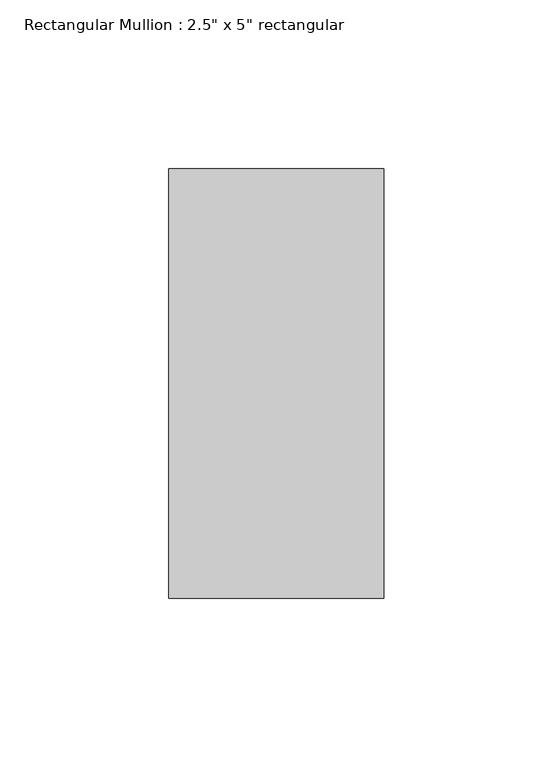
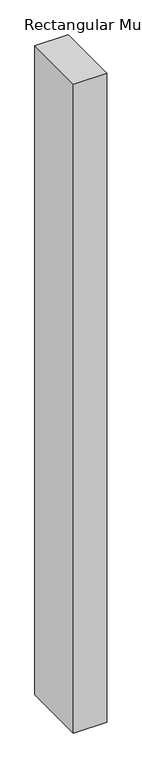
"""IFC4 building model written with IfcOpenShell, lengths in millimetres: member geometry."""

from ifc_helpers import new_model, si_unit, frame, origin, place, context, project, spatial, polyline, outline, extrude, source, transform, mapped, element, save


def member_8eff11ef(model_context):
    return source(origin(), model_context, "Body", "SweptSolid", [
        extrude(outline(polyline([(0.0, 63.5), (0.0, -63.5), (-63.5, -63.5), (-63.5, 63.5), (0.0, 63.5)])), frame((0.0, 0.0, -1308.0999998), z_axis=(0.0, 0.0, 1.0), x_axis=(1.0, 0.0, 0.0)), (0.0, 0.0, 1.0), 1308.0999998),
    ])


if __name__ == "__main__":
    model = new_model("IFC4")
    model_context = context("Model", 3, world=origin())
    ifc_project = project(units=[si_unit("LENGTHUNIT", "METRE", prefix="MILLI")], contexts=[model_context])
    site = spatial("IfcSite", under=ifc_project)
    building = spatial("IfcBuilding", under=site)
    placement = place(None, origin())
    member_shape = member_8eff11ef(model_context)
    element("IfcMember", 1, ObjectType="Rectangular Mullion : 2.5\" x 5\" rectangular", at=placement, inside=building, context=model_context, shape_type="MappedRepresentation", body=[
        mapped(member_shape, transform((0.0, 0.0, 0.0), x_axis=(1.0, 0.0, 0.0), y_axis=(0.0, 1.0, 0.0), z_axis=(0.0, 0.0, 1.0))),
    ])
    save(model, "model.ifc")

# Revit data of these elements
# Type "Rectangular Mullion : 2.5\" x 5\" rectangular"
#   built-in parameter 1007304 = 0.416667 (stored number, unit not read)
#   built-in parameter 1007301 = 0.104167 (stored number, unit not read)
#   built-in parameter 1007300 = 0.104167 (stored number, unit not read)
# Element 1 (IfcMember, "Rectangular Mullion : 2.5\" x 5\" rectangular")
#   Materials on its faces: "Aluminum"
# Materials
#   "Aluminum": class "Metal", colour RGB 247 247 247, transparency 0, Description = "Aluminum 6061", Cost = 0
